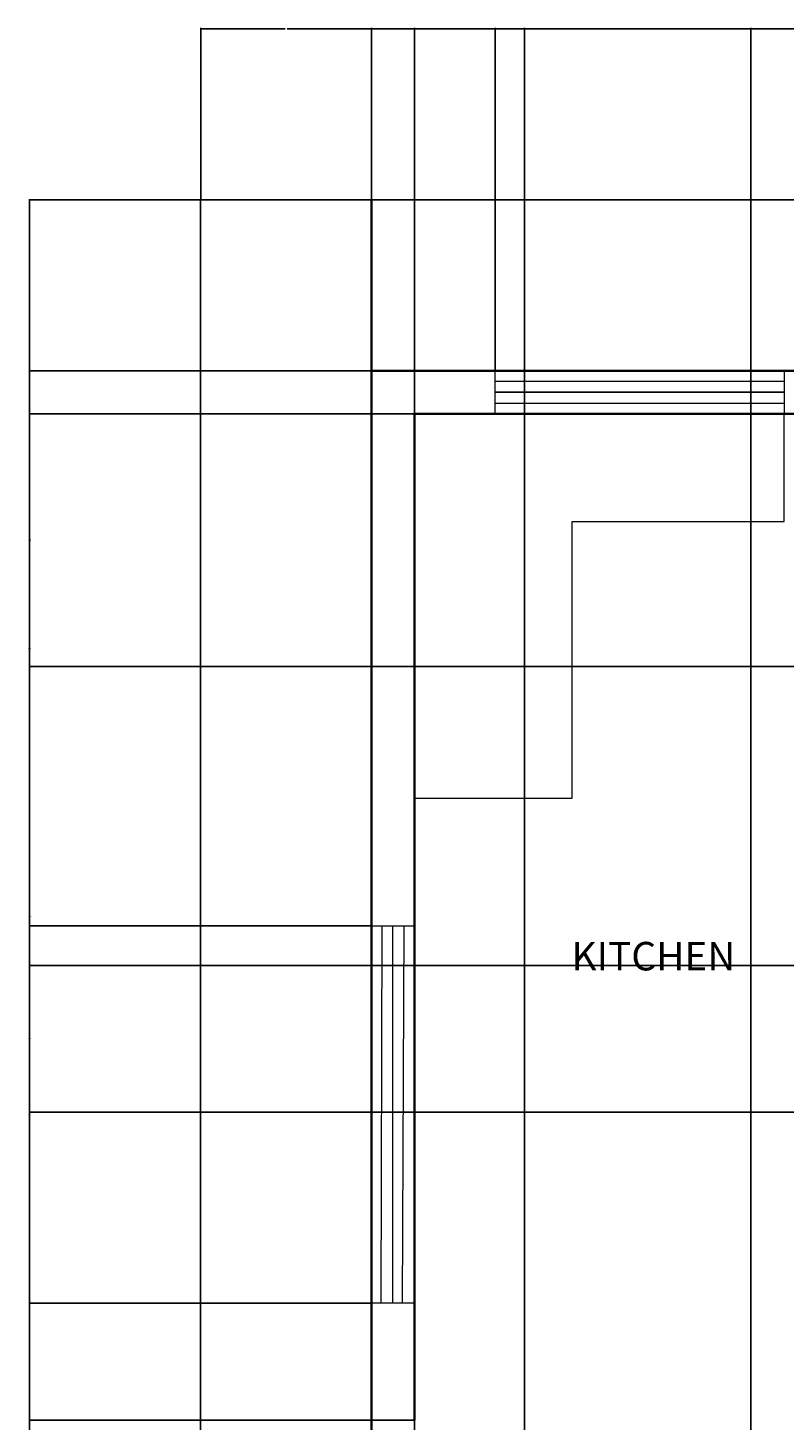
# Model space of a CAD drawing. Units: inches. Extents: x 2621 to 3621, y 1701 to 2465.
# Tile 3 of 6: x 2621 to 2780, y 2169 to 2462. Entities that reach past the tile are written whole.
import ezdxf

# ---------------------------------------------------------------- set-up
doc = ezdxf.new("R2010")
doc.units = ezdxf.units.IN
for name, color, linetype, lineweight in [('A-ANNO-DIMS', 2, 'Continuous', 18), ('A-AREA-IDEN', 7, 'Continuous', 18), ('A-FLOR-CASE', 32, 'Continuous', 18), ('A-GLAZ', 4, 'Continuous', 18), ('A-WALL', 7, 'Continuous', 35), ('C-PROP', 8, 'Continuous', 25)]:
    doc.layers.add(name, color=color, linetype=linetype, lineweight=lineweight)
doc.styles.get("Standard").update_dxf_attribs({"font": 'arial.ttf'})
doc.dimstyles.get("Standard").update_dxf_attribs({"dimtxt": 0.18, "dimasz": 0.18, "dimexe": 0.18, "dimexo": 0.0625, "dimgap": 0.09, "dimtad": 0, "dimtih": 1, "dimtoh": 1, "dimdec": 4, "dimzin": 0, "dimdsep": 46, "dimtxsty": 'Standard', "dimcen": 0.09, "dimadec": 0, "dimazin": 0, "dimtfac": 1, "dimtdec": 4, "dimtofl": 0, "dimtmove": 0, "dimatfit": 3, "dimfxl": 1, "dimtolj": 1, "dimtzin": 0, "dimarcsym": 0})

# ---------------------------------------------------------------- blocks, each defined once
blk = doc.blocks.new('LOT-33X57')
for p, q in [((0, 684), (396, 684)), ((0, 0), (0, 684))]:
    blk.add_line(p, q)
blk = doc.blocks.new('WIN-60_89')
for p, q in [((0, 6.86), (60.89, 6.86)), ((0, 2.21), (60.89, 2.21))]:
    blk.add_line(p, q)
for points in [[(0, 9), (60.89, 9), (60.89, 0), (0, 0)], [(0, 4.5), (60.89, 4.5), (60.89, 4.5), (0, 4.5)]]:
    blk.add_lwpolyline(points, close=True)
blk = doc.blocks.new('*D36')
at = {"layer": 'A-ANNO-DIMS', "color": 0, "lineweight": -2, "transparency": 16777216}
for p, q in [((2657.46, 2425.4), (2621.31, 2425.4)), ((2621.49, 2425.22), (2621.49, 2083.58)), ((2621.49, 1741.58), (2621.49, 2083.22)), ((2657.46, 1741.4), (2621.31, 1741.4))]:
    blk.add_line(p, q, dxfattribs=at)
at = {"layer": 'A-ANNO-DIMS', "color": 0, "transparency": 16777216}
for points in [[(2621.46, 2425.22), (2621.52, 2425.22), (2621.49, 2425.4)], [(2621.46, 1741.58), (2621.52, 1741.58), (2621.49, 1741.4)]]:
    blk.add_solid(points, dxfattribs=at)
at = {"layer": 'Defpoints', "color": 0, "transparency": 16777216}
for p in [(2621.49, 2425.4), (2657.52, 2425.4), (2657.52, 1741.4)]:
    blk.add_point(p, dxfattribs=at)
at = {"layer": 'A-ANNO-DIMS', "color": 0, "transparency": 16777216, "insert": (2621.49, 2083.4), "char_height": 0.18, "attachment_point": 5}
blk.add_mtext('\\A1;684', dxfattribs=at)
blk = doc.blocks.new('*D37')
at = {"layer": 'A-ANNO-DIMS', "color": 0, "lineweight": -2, "transparency": 16777216}
for p, q in [((2693.52, 2425.46), (2693.52, 2461.61)), ((3039.37, 2204.63), (3039.37, 2461.61)), ((2693.7, 2461.43), (2865.98, 2461.43)), ((3039.19, 2461.43), (2866.91, 2461.43))]:
    blk.add_line(p, q, dxfattribs=at)
at = {"layer": 'A-ANNO-DIMS', "color": 0, "transparency": 16777216}
for points in [[(2693.7, 2461.46), (2693.7, 2461.4), (2693.52, 2461.43)], [(3039.19, 2461.46), (3039.19, 2461.4), (3039.37, 2461.43)]]:
    blk.add_solid(points, dxfattribs=at)
at = {"layer": 'Defpoints', "color": 0, "transparency": 16777216}
for p in [(3039.37, 2461.43), (2693.52, 2425.4), (3039.37, 2204.57)]:
    blk.add_point(p, dxfattribs=at)
at = {"layer": 'A-ANNO-DIMS', "color": 0, "transparency": 16777216, "insert": (2866.44, 2461.43), "char_height": 0.18, "attachment_point": 5}
blk.add_mtext('\\A1;345.85', dxfattribs=at)
blk = doc.blocks.new('*D39')
at = {"layer": 'A-ANNO-DIMS', "color": 0, "lineweight": -2, "transparency": 16777216}
for p, q in [((2657.52, 2425.46), (2657.52, 2461.61)), ((2693.52, 2425.46), (2693.52, 2461.61)), ((2657.7, 2461.43), (2675.3, 2461.43)), ((2693.34, 2461.43), (2675.74, 2461.43))]:
    blk.add_line(p, q, dxfattribs=at)
at = {"layer": 'A-ANNO-DIMS', "color": 0, "transparency": 16777216}
for points in [[(2657.7, 2461.46), (2657.7, 2461.4), (2657.52, 2461.43)], [(2693.34, 2461.46), (2693.34, 2461.4), (2693.52, 2461.43)]]:
    blk.add_solid(points, dxfattribs=at)
at = {"layer": 'Defpoints', "color": 0, "transparency": 16777216}
for p in [(2693.52, 2461.43), (2657.52, 2425.4), (2693.52, 2425.4)]:
    blk.add_point(p, dxfattribs=at)
at = {"layer": 'A-ANNO-DIMS', "color": 0, "transparency": 16777216, "insert": (2675.52, 2461.43), "char_height": 0.18, "attachment_point": 5}
blk.add_mtext('\\A1;36', dxfattribs=at)
blk = doc.blocks.new('*D41')
at = {"layer": 'A-ANNO-DIMS', "color": 0, "lineweight": -2, "transparency": 16777216}
for p, q in [((2693.58, 2425.4), (3089.72, 2425.4)), ((3089.54, 2425.22), (3089.54, 2407.58)), ((3089.54, 2389.58), (3089.54, 2407.22)), ((2693.58, 2389.4), (3089.72, 2389.4))]:
    blk.add_line(p, q, dxfattribs=at)
at = {"layer": 'A-ANNO-DIMS', "color": 0, "transparency": 16777216}
for points in [[(3089.51, 2425.22), (3089.57, 2425.22), (3089.54, 2425.4)], [(3089.51, 2389.58), (3089.57, 2389.58), (3089.54, 2389.4)]]:
    blk.add_solid(points, dxfattribs=at)
at = {"layer": 'Defpoints', "color": 0, "transparency": 16777216}
for p in [(2693.52, 2425.4), (2693.52, 2389.4), (3089.54, 2389.4)]:
    blk.add_point(p, dxfattribs=at)
at = {"layer": 'A-ANNO-DIMS', "color": 0, "transparency": 16777216, "insert": (3089.54, 2407.4), "char_height": 0.18, "attachment_point": 5}
blk.add_mtext('\\A1;36', dxfattribs=at)
blk = doc.blocks.new('*D42')
at = {"layer": 'A-ANNO-DIMS', "color": 0, "lineweight": -2, "transparency": 16777216}
for p, q in [((2702.52, 2380.34), (2702.52, 1705.2)), ((2809.02, 2380.34), (2809.02, 1705.2)), ((2702.7, 1705.38), (2755.38, 1705.38)), ((2808.84, 1705.38), (2756.15, 1705.38))]:
    blk.add_line(p, q, dxfattribs=at)
at = {"layer": 'A-ANNO-DIMS', "color": 0, "transparency": 16777216}
for points in [[(2702.7, 1705.41), (2702.7, 1705.35), (2702.52, 1705.38)], [(2808.84, 1705.41), (2808.84, 1705.35), (2809.02, 1705.38)]]:
    blk.add_solid(points, dxfattribs=at)
at = {"layer": 'Defpoints', "color": 0, "transparency": 16777216}
for p in [(2702.52, 2380.4), (2809.02, 2380.4), (2809.02, 1705.38)]:
    blk.add_point(p, dxfattribs=at)
at = {"layer": 'A-ANNO-DIMS', "color": 0, "transparency": 16777216, "insert": (2755.77, 1705.38), "char_height": 0.18, "attachment_point": 5}
blk.add_mtext('\\A1;106.5', dxfattribs=at)
blk = doc.blocks.new('*D48')
at = {"layer": 'A-ANNO-DIMS', "color": 0, "lineweight": -2, "transparency": 16777216}
for p, q in [((2702.46, 2380.4), (2621.31, 2380.4)), ((2621.49, 2380.22), (2621.49, 2274.67)), ((2621.49, 2168.75), (2621.49, 2274.3)), ((2702.46, 2168.57), (2621.31, 2168.57))]:
    blk.add_line(p, q, dxfattribs=at)
at = {"layer": 'A-ANNO-DIMS', "color": 0, "transparency": 16777216}
for points in [[(2621.46, 2380.22), (2621.52, 2380.22), (2621.49, 2380.4)], [(2621.46, 2168.75), (2621.52, 2168.75), (2621.49, 2168.57)]]:
    blk.add_solid(points, dxfattribs=at)
at = {"layer": 'Defpoints', "color": 0, "transparency": 16777216}
for p in [(2621.49, 2380.4), (2702.52, 2380.4), (2702.52, 2168.57)]:
    blk.add_point(p, dxfattribs=at)
at = {"layer": 'A-ANNO-DIMS', "color": 0, "transparency": 16777216, "insert": (2621.49, 2274.49), "char_height": 0.18, "attachment_point": 5}
blk.add_mtext('\\A1;211.83', dxfattribs=at)
blk = doc.blocks.new('*D52')
at = {"layer": 'A-ANNO-DIMS', "color": 0, "lineweight": -2, "transparency": 16777216}
for p, q in [((2702.52, 1892.46), (2702.52, 2461.61)), ((2884, 1887.96), (2884, 2461.61)), ((2702.7, 2461.43), (2792.8, 2461.43)), ((2883.82, 2461.43), (2793.71, 2461.43))]:
    blk.add_line(p, q, dxfattribs=at)
at = {"layer": 'A-ANNO-DIMS', "color": 0, "transparency": 16777216}
for points in [[(2702.7, 2461.46), (2702.7, 2461.4), (2702.52, 2461.43)], [(2883.82, 2461.46), (2883.82, 2461.4), (2884, 2461.43)]]:
    blk.add_solid(points, dxfattribs=at)
at = {"layer": 'Defpoints', "color": 0, "transparency": 16777216}
for p in [(2884, 2461.43), (2702.52, 1892.4), (2884, 1887.9)]:
    blk.add_point(p, dxfattribs=at)
at = {"layer": 'A-ANNO-DIMS', "color": 0, "transparency": 16777216, "insert": (2793.26, 2461.43), "char_height": 0.18, "attachment_point": 5}
blk.add_mtext('\\A1;181.48', dxfattribs=at)
blk = doc.blocks.new('*D81')
at = {"layer": 'A-ANNO-DIMS', "color": 0, "lineweight": -2, "transparency": 16777216}
for p, q in [((2693.52, 2389.46), (2693.52, 2461.61)), ((2719.52, 2389.46), (2719.52, 2461.61)), ((2693.7, 2461.43), (2706.05, 2461.43)), ((2719.34, 2461.43), (2706.98, 2461.43))]:
    blk.add_line(p, q, dxfattribs=at)
at = {"layer": 'A-ANNO-DIMS', "color": 0, "transparency": 16777216}
for points in [[(2693.7, 2461.46), (2693.7, 2461.4), (2693.52, 2461.43)], [(2719.34, 2461.46), (2719.34, 2461.4), (2719.52, 2461.43)]]:
    blk.add_solid(points, dxfattribs=at)
at = {"layer": 'Defpoints', "color": 0, "transparency": 16777216}
for p in [(2719.52, 2461.43), (2693.52, 2389.4), (2719.52, 2389.4)]:
    blk.add_point(p, dxfattribs=at)
at = {"layer": 'A-ANNO-DIMS', "color": 0, "transparency": 16777216, "insert": (2706.52, 2461.43), "char_height": 0.18, "attachment_point": 5}
blk.add_mtext('\\A1;25.997', dxfattribs=at)
blk = doc.blocks.new('*D85')
at = {"layer": 'A-ANNO-DIMS', "color": 0, "lineweight": -2, "transparency": 16777216}
for p, q in [((2693.46, 2389.4), (2621.31, 2389.4)), ((2621.49, 2389.22), (2621.49, 2331.19)), ((2621.49, 2272.8), (2621.49, 2330.83)), ((2693.46, 2272.62), (2621.31, 2272.62))]:
    blk.add_line(p, q, dxfattribs=at)
at = {"layer": 'A-ANNO-DIMS', "color": 0, "transparency": 16777216}
for points in [[(2621.46, 2389.22), (2621.52, 2389.22), (2621.49, 2389.4)], [(2621.46, 2272.8), (2621.52, 2272.8), (2621.49, 2272.62)]]:
    blk.add_solid(points, dxfattribs=at)
at = {"layer": 'Defpoints', "color": 0, "transparency": 16777216}
for p in [(2621.49, 2389.4), (2693.52, 2389.4), (2693.52, 2272.62)]:
    blk.add_point(p, dxfattribs=at)
at = {"layer": 'A-ANNO-DIMS', "color": 0, "transparency": 16777216, "insert": (2621.49, 2331.01), "char_height": 0.18, "attachment_point": 5}
blk.add_mtext('\\A1;116.78', dxfattribs=at)
blk = doc.blocks.new('*D86')
at = {"layer": 'A-ANNO-DIMS', "color": 0, "lineweight": -2, "transparency": 16777216}
for p, q in [((2693.46, 2272.62), (2621.31, 2272.62)), ((2621.49, 2272.44), (2621.49, 2233.09)), ((2621.49, 2193.39), (2621.49, 2232.73)), ((2693.46, 2193.21), (2621.31, 2193.21))]:
    blk.add_line(p, q, dxfattribs=at)
at = {"layer": 'A-ANNO-DIMS', "color": 0, "transparency": 16777216}
for points in [[(2621.46, 2272.44), (2621.52, 2272.44), (2621.49, 2272.62)], [(2621.46, 2193.39), (2621.52, 2193.39), (2621.49, 2193.21)]]:
    blk.add_solid(points, dxfattribs=at)
at = {"layer": 'Defpoints', "color": 0, "transparency": 16777216}
for p in [(2621.49, 2272.62), (2693.52, 2272.62), (2693.52, 2193.21)]:
    blk.add_point(p, dxfattribs=at)
at = {"layer": 'A-ANNO-DIMS', "color": 0, "transparency": 16777216, "insert": (2621.49, 2232.91), "char_height": 0.18, "attachment_point": 5}
blk.add_mtext('\\A1;79.41', dxfattribs=at)
blk = doc.blocks.new('*D91')
at = {"layer": 'A-ANNO-DIMS', "color": 0, "lineweight": -2, "transparency": 16777216}
for p, q in [((3008.46, 2380.4), (2621.31, 2380.4)), ((2621.49, 2380.22), (2621.49, 2353.98)), ((2621.49, 2327.37), (2621.49, 2353.61)), ((3008.46, 2327.19), (2621.31, 2327.19))]:
    blk.add_line(p, q, dxfattribs=at)
at = {"layer": 'A-ANNO-DIMS', "color": 0, "transparency": 16777216}
for points in [[(2621.46, 2380.22), (2621.52, 2380.22), (2621.49, 2380.4)], [(2621.46, 2327.37), (2621.52, 2327.37), (2621.49, 2327.19)]]:
    blk.add_solid(points, dxfattribs=at)
at = {"layer": 'Defpoints', "color": 0, "transparency": 16777216}
for p in [(2621.49, 2380.4), (3008.52, 2380.4), (3008.52, 2327.19)]:
    blk.add_point(p, dxfattribs=at)
at = {"layer": 'A-ANNO-DIMS', "color": 0, "transparency": 16777216, "insert": (2621.49, 2353.79), "char_height": 0.18, "attachment_point": 5}
blk.add_mtext('\\A1;53.22', dxfattribs=at)
blk = doc.blocks.new('*D98')
at = {"layer": 'A-ANNO-DIMS', "color": 0, "lineweight": -2, "transparency": 16777216}
for p, q in [((2702.52, 1892.46), (2702.52, 2461.61)), ((2725.71, 1892.46), (2725.71, 2461.61)), ((2702.7, 2461.43), (2713.72, 2461.43)), ((2725.53, 2461.43), (2714.51, 2461.43))]:
    blk.add_line(p, q, dxfattribs=at)
at = {"layer": 'A-ANNO-DIMS', "color": 0, "transparency": 16777216}
for points in [[(2702.7, 2461.46), (2702.7, 2461.4), (2702.52, 2461.43)], [(2725.53, 2461.46), (2725.53, 2461.4), (2725.71, 2461.43)]]:
    blk.add_solid(points, dxfattribs=at)
at = {"layer": 'Defpoints', "color": 0, "transparency": 16777216}
for p in [(2725.71, 2461.43), (2702.52, 1892.4), (2725.71, 1892.4)]:
    blk.add_point(p, dxfattribs=at)
at = {"layer": 'A-ANNO-DIMS', "color": 0, "transparency": 16777216, "insert": (2714.11, 2461.43), "char_height": 0.18, "attachment_point": 5}
blk.add_mtext('\\A1;23.19', dxfattribs=at)
blk = doc.blocks.new('*D99')
at = {"layer": 'A-ANNO-DIMS', "color": 0, "lineweight": -2, "transparency": 16777216}
for p, q in [((2725.71, 1892.46), (2725.71, 2461.61)), ((2773.36, 1892.46), (2773.36, 2461.61)), ((2725.89, 2461.43), (2749.13, 2461.43)), ((2773.18, 2461.43), (2749.93, 2461.43))]:
    blk.add_line(p, q, dxfattribs=at)
at = {"layer": 'A-ANNO-DIMS', "color": 0, "transparency": 16777216}
for points in [[(2725.89, 2461.46), (2725.89, 2461.4), (2725.71, 2461.43)], [(2773.18, 2461.46), (2773.18, 2461.4), (2773.36, 2461.43)]]:
    blk.add_solid(points, dxfattribs=at)
at = {"layer": 'Defpoints', "color": 0, "transparency": 16777216}
for p in [(2773.36, 2461.43), (2725.71, 1892.4), (2773.36, 1892.4)]:
    blk.add_point(p, dxfattribs=at)
at = {"layer": 'A-ANNO-DIMS', "color": 0, "transparency": 16777216, "insert": (2749.53, 2461.43), "char_height": 0.18, "attachment_point": 5}
blk.add_mtext('\\A1;47.65', dxfattribs=at)
blk = doc.blocks.new('*D101')
at = {"layer": 'A-ANNO-DIMS', "color": 0, "lineweight": -2, "transparency": 16777216}
for p, q in [((2808.96, 2264.26), (2621.31, 2264.26)), ((2621.49, 2264.08), (2621.49, 2248.99)), ((2621.49, 2233.55), (2621.49, 2248.63)), ((2808.96, 2233.37), (2621.31, 2233.37))]:
    blk.add_line(p, q, dxfattribs=at)
at = {"layer": 'A-ANNO-DIMS', "color": 0, "transparency": 16777216}
for points in [[(2621.46, 2264.08), (2621.52, 2264.08), (2621.49, 2264.26)], [(2621.46, 2233.55), (2621.52, 2233.55), (2621.49, 2233.37)]]:
    blk.add_solid(points, dxfattribs=at)
at = {"layer": 'Defpoints', "color": 0, "transparency": 16777216}
for p in [(2621.49, 2264.26), (2809.02, 2264.26), (2809.02, 2233.37)]:
    blk.add_point(p, dxfattribs=at)
at = {"layer": 'A-ANNO-DIMS', "color": 0, "transparency": 16777216, "insert": (2621.49, 2248.81), "char_height": 0.18, "attachment_point": 5}
blk.add_mtext('\\A1;30.896', dxfattribs=at)

msp = doc.modelspace()

# ---------------------------------------------------------------- linework, layer by layer
at = {"layer": 'A-FLOR-CASE'}
for p, q in [((2780.4086, 2357.7135), (2780.4086, 2380.4015)), ((2735.7748, 2299.4879), (2735.7748, 2357.7135)), ((2735.7748, 2357.7135), (2780.4086, 2357.7135)), ((2702.5184, 2299.4879), (2735.7748, 2299.4879))]:
    msp.add_line(p, q, dxfattribs=at)
at = {"layer": 'A-GLAZ'}
for p, q in [((2695.5329, 2193.2066), (2695.7745, 2272.6181)), ((2698.0184, 2193.2066), (2698.0184, 2272.6181)), ((2700.004, 2193.2066), (2700.3665, 2272.6181))]:
    msp.add_line(p, q, dxfattribs=at)
msp.add_lwpolyline([(2693.5184, 2272.6181), (2702.5184, 2272.6181), (2702.5184, 2193.2066), (2693.5184, 2193.2066)], close=True, dxfattribs=at)
at = {"layer": 'A-WALL'}
for p, q in [((2693.5184, 2425.4015), (2693.5184, 1887.8987)), ((3017.5184, 2389.4015), (2693.5184, 2389.4015)), ((2702.5184, 2380.4015), (2702.5184, 2168.5709)), ((2809.0179, 2380.4015), (2702.5184, 2380.4015))]:
    msp.add_line(p, q, dxfattribs=at)

# ---------------------------------------------------------------- block references
at = {"layer": 'A-GLAZ'}
msp.add_blockref('WIN-60_89', (2719.516, 2380.402), dxfattribs=at)
at = {"layer": 'C-PROP'}
msp.add_blockref('LOT-33X57', (2657.518, 1741.402), dxfattribs=at)

# ---------------------------------------------------------------- texts
at = {"layer": 'A-AREA-IDEN', "insert": (2735.6259, 2269.2256), "char_height": 6, "attachment_point": 1}
msp.add_mtext_dynamic_manual_height_columns('KITCHEN ', width=42.031369, gutter_width=12.5, heights=[0], dxfattribs=at)

# ---------------------------------------------------------------- dimensions: what is measured, and where the dimension line sits
at = {"layer": 'A-ANNO-DIMS'}
for base, p1, p2, override, picture, middle in [((2693.5184, 2461.427), (2657.5184, 2425.4015), (2693.5184, 2425.4015), {"dimdec": 0, "dimlfac": 1, "dimrnd": 0, "dimzin": 0, "dimdsep": 46, "dimlunit": 2}, '*D39', (2675.5184, 2461.427)), ((3039.3697, 2461.427), (2693.5184, 2425.4015), (3039.3697, 2204.5707), {"dimdec": 2, "dimlfac": 1, "dimrnd": 0, "dimzin": 0, "dimdsep": 46, "dimlunit": 2}, '*D37', (2866.444, 2461.427)), ((2719.5156, 2461.427), (2693.5184, 2389.4015), (2719.5156, 2389.4015), {"dimdec": 3, "dimlfac": 1, "dimrnd": 0, "dimzin": 0, "dimdsep": 46, "dimlunit": 2}, '*D81', (2706.517, 2461.427)), ((2883.995, 2461.427), (2702.5184, 1892.3987), (2883.995, 1887.8987), {"dimdec": 2, "dimlfac": 1, "dimrnd": 0, "dimzin": 0, "dimdsep": 46, "dimlunit": 2}, '*D52', (2793.2567, 2461.427)), ((2725.7097, 2461.427), (2702.5184, 1892.3987), (2725.7097, 1892.3987), {"dimdec": 2, "dimlfac": 1, "dimrnd": 0, "dimzin": 0, "dimdsep": 46, "dimlunit": 2}, '*D98', (2714.114, 2461.427)), ((2773.3557, 2461.427), (2725.7097, 1892.3987), (2773.3557, 1892.3987), {"dimdec": 2, "dimlfac": 1, "dimrnd": 0, "dimzin": 0, "dimdsep": 46, "dimlunit": 2}, '*D99', (2749.5327, 2461.427)), ((2809.0179, 1705.376), (2702.5184, 2380.4015), (2809.0179, 2380.4015), {"dimdec": 1, "dimlfac": 1, "dimrnd": 0, "dimzin": 0, "dimdsep": 46, "dimlunit": 2}, '*D42', (2755.7681, 1705.376))]:
    dim = msp.add_linear_dim(base=base, p1=p1, p2=p2, dimstyle='Standard', override=override, dxfattribs=at)
    dim.commit()
    dim.dimension.update_dxf_attribs({"geometry": picture, "text_midpoint": middle})
for base, p1, p2, override, picture, middle in [((2621.4929, 2425.4015), (2657.5184, 1741.4015), (2657.5184, 2425.4015), {"dimdec": 0, "dimlfac": 1, "dimrnd": 0, "dimzin": 0, "dimdsep": 46, "dimlunit": 2}, '*D36', (2621.4929, 2083.4015)), ((3089.5439, 2389.4015), (2693.5184, 2425.4015), (2693.5184, 2389.4015), {"dimdec": 0, "dimlfac": 1, "dimrnd": 0, "dimzin": 0, "dimdsep": 46, "dimlunit": 2}, '*D41', (3089.5439, 2407.4015)), ((2621.4929, 2389.4015), (2693.5184, 2272.6181), (2693.5184, 2389.4015), {"dimdec": 2, "dimlfac": 1, "dimrnd": 0, "dimzin": 0, "dimdsep": 46, "dimlunit": 2}, '*D85', (2621.4929, 2331.0098)), ((2621.4929, 2380.4015), (2702.5184, 2168.5709), (2702.5184, 2380.4015), {"dimdec": 2, "dimlfac": 1, "dimrnd": 0, "dimzin": 0, "dimdsep": 46, "dimlunit": 2}, '*D48', (2621.4929, 2274.4862)), ((2621.4929, 2380.4015), (3008.5184, 2327.1855), (3008.5184, 2380.4015), {"dimdec": 2, "dimlfac": 1, "dimrnd": 0, "dimzin": 0, "dimdsep": 46, "dimlunit": 2}, '*D91', (2621.4929, 2353.7935)), ((2621.4929, 2272.6181), (2693.5184, 2193.2066), (2693.5184, 2272.6181), {"dimdec": 2, "dimlfac": 1, "dimrnd": 0, "dimzin": 0, "dimdsep": 46, "dimlunit": 2}, '*D86', (2621.4929, 2232.9123)), ((2621.4929, 2264.2608), (2809.0179, 2233.3652), (2809.0179, 2264.2608), {"dimdec": 3, "dimlfac": 1, "dimrnd": 0, "dimzin": 0, "dimdsep": 46, "dimlunit": 2}, '*D101', (2621.4929, 2248.813))]:
    dim = msp.add_linear_dim(base=base, p1=p1, p2=p2, angle=90, dimstyle='Standard', override=override, dxfattribs=at)
    dim.commit()
    dim.dimension.update_dxf_attribs({"geometry": picture, "text_midpoint": middle})

doc.saveas('drawing.dxf')
